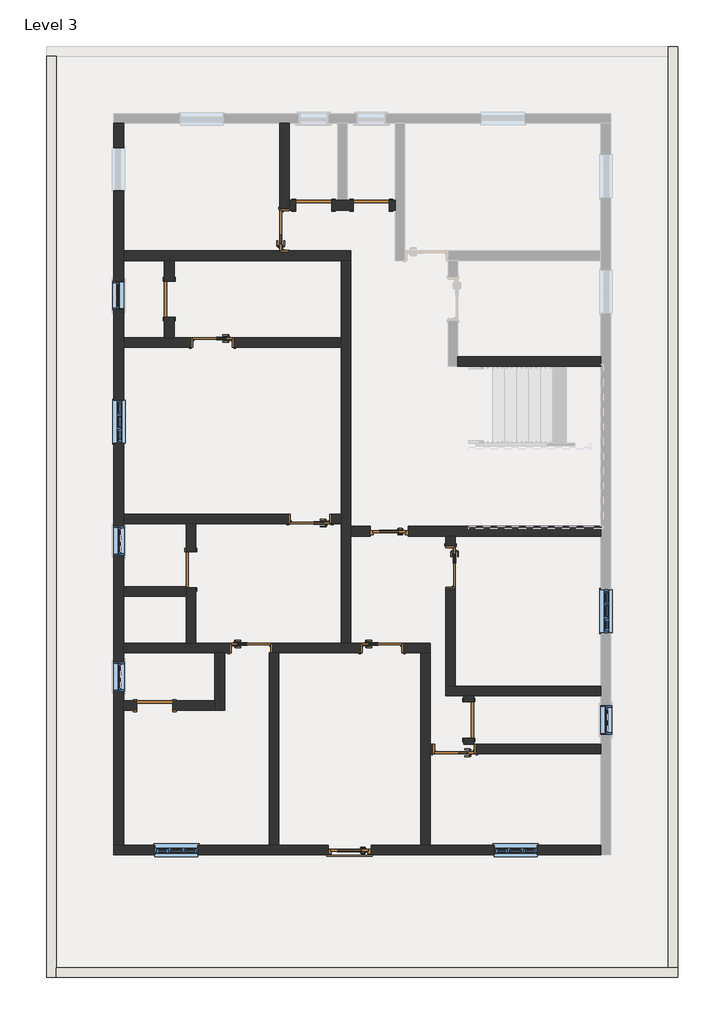
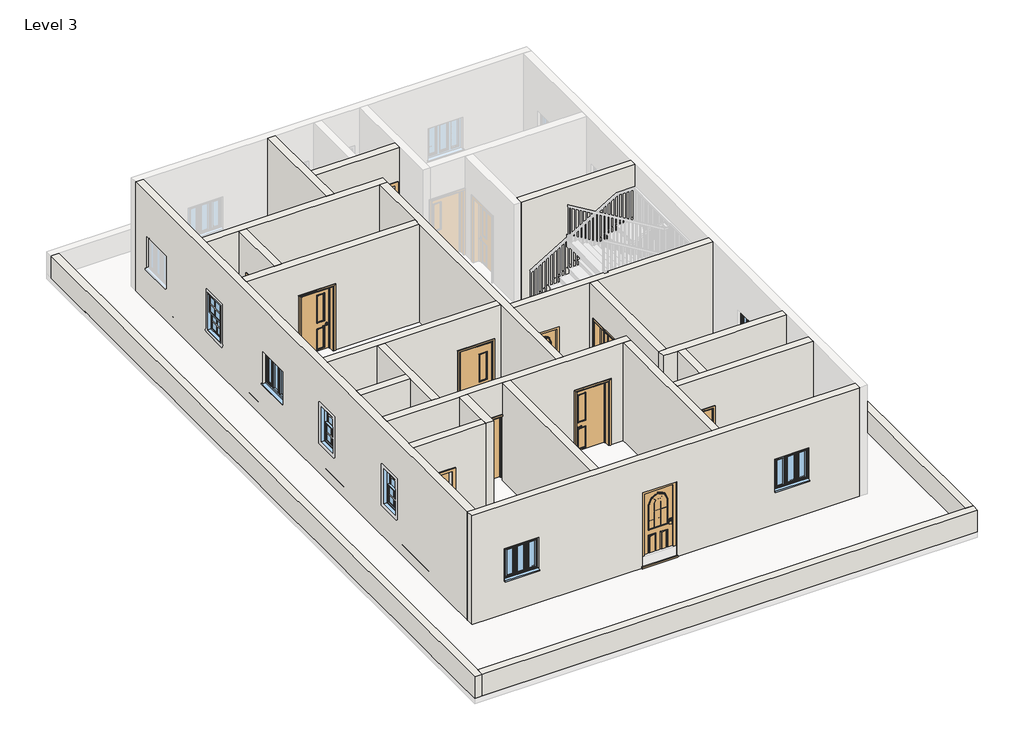
# One storey, part 1 of 3: 25 walls, 15 doors, 8 windows.
"""IFC4 building model written with IfcOpenShell, lengths in millimetres."""

from ifc_helpers import new_model, si_unit, frame, origin, place, context, project, spatial, polyline, outline, extrude, faceted_brep, transform, mapped, element, save
from components import doors_extsgl_w_glazing_bars_arched_810x2110mm_57ea6d9e, doors_extsgl_w_glazing_bars_arched_910x2110mm_1ab485ba, door_aa1d4bf3, door_2f4bc105, door_fadea3f2, door_53b1b562, window_679d2811, windows_tpl_w_glazing_bars_910x910mm_9d987a72

model = new_model("IFC4")

# Units and contexts
model_context = context("Model", 3, world=origin())
ifc_project = project(units=[si_unit("LENGTHUNIT", "METRE", prefix="MILLI")], contexts=[model_context])

# Site, building, storey
site = spatial("IfcSite", under=ifc_project)
building = spatial("IfcBuilding", under=site)
storey = spatial("IfcBuildingStorey", under=building, Name="Level 3", Elevation=6096.0)

# Doors
placement = place(None, origin())
doors_extsgl_w_glazing_bars_arched_810x2110mm_shape = doors_extsgl_w_glazing_bars_arched_810x2110mm_57ea6d9e(model_context)
element("IfcDoor", 1, ObjectType="Doors_ExtSgl_w-Glazing_Bars_Arched : 810x2110mm", at=placement, inside=storey, context=model_context, shape_type="MappedRepresentation", body=[
    mapped(doors_extsgl_w_glazing_bars_arched_810x2110mm_shape, transform((-8090.5711241, 8252.7344295, 6096.0), x_axis=(-1.0, 0.0, 0.0), y_axis=(0.0, -1.0, 0.0), z_axis=(0.0, 0.0, 1.0))),
])
doors_extsgl_w_glazing_bars_arched_910x2110mm_shape = doors_extsgl_w_glazing_bars_arched_910x2110mm_1ab485ba(model_context)
element("IfcDoor", 2, ObjectType="Doors_ExtSgl_w-Glazing_Bars_Arched : 910x2110mm", at=placement, inside=storey, context=model_context, shape_type="MappedRepresentation", body=[
    mapped(doors_extsgl_w_glazing_bars_arched_910x2110mm_shape, transform((-8928.7711241, 1521.7344295, 6096.0), x_axis=(-1.0, 0.0, 0.0), y_axis=(0.0, -1.0, 0.0), z_axis=(0.0, 0.0, 1.0))),
])
door_shape = door_aa1d4bf3(model_context)
element("IfcDoor", 3, ObjectType="Doors_IntSgl_3 : 7'-3\"", at=placement, inside=storey, context=model_context, shape_type="MappedRepresentation", body=[
    mapped(door_shape, transform((-10300.3711241, 14602.7344295, 6096.0), x_axis=(0.0, 1.0, 0.0), y_axis=(-1.0, 0.0, 0.0), z_axis=(0.0, 0.0, 1.0))),
])
element("IfcDoor", 4, ObjectType="Doors_IntSgl_3 : 7'-3\"", at=placement, inside=storey, context=model_context, shape_type="MappedRepresentation", body=[
    mapped(door_shape, transform((-8242.9711241, 5788.9344295, 6096.0), x_axis=(1.0, 0.0, 0.0), y_axis=(0.0, 1.0, 0.0), z_axis=(0.0, 0.0, 1.0))),
])
element("IfcDoor", 5, ObjectType="Doors_IntSgl_3 : 7'-3\"", at=placement, inside=storey, context=model_context, shape_type="MappedRepresentation", body=[
    mapped(door_shape, transform((-6795.1711241, 7490.7344295, 6096.0), x_axis=(0.0, -1.0, 0.0), y_axis=(1.0, 0.0, 0.0), z_axis=(0.0, 0.0, 1.0))),
])
element("IfcDoor", 6, ObjectType="Doors_IntSgl_3 : 7'-3\"", at=placement, inside=storey, context=model_context, shape_type="MappedRepresentation", body=[
    mapped(door_shape, transform((-11011.5711241, 5788.9344295, 6096.0), x_axis=(1.0, 0.0, 0.0), y_axis=(0.0, 1.0, 0.0), z_axis=(0.0, 0.0, 1.0))),
])
element("IfcDoor", 7, ObjectType="Doors_IntSgl_3 : 7'-3\"", at=placement, inside=storey, context=model_context, shape_type="MappedRepresentation", body=[
    mapped(door_shape, transform((-9766.9711241, 8506.7344295, 6096.0), x_axis=(-1.0, 0.0, 0.0), y_axis=(0.0, -1.0, 0.0), z_axis=(0.0, 0.0, 1.0))),
])
element("IfcDoor", 8, ObjectType="Doors_IntSgl_3 : 7'-3\"", at=placement, inside=storey, context=model_context, shape_type="MappedRepresentation", body=[
    mapped(door_shape, transform((-6718.9711241, 3655.3344295, 6096.0), x_axis=(-1.0, 0.0, 0.0), y_axis=(0.0, -1.0, 0.0), z_axis=(0.0, 0.0, 1.0))),
])
door_2_shape = door_2f4bc105(model_context)
element("IfcDoor", 9, ObjectType="Doors_IntSgl_3 : 7'-3\"", at=placement, inside=storey, context=model_context, shape_type="MappedRepresentation", body=[
    mapped(door_2_shape, transform((-11824.3711241, 12240.5344295, 6096.0), x_axis=(-1.0, 0.0, 0.0), y_axis=(0.0, -1.0, 0.0), z_axis=(0.0, 0.0, 1.0))),
])
door_3_shape = door_fadea3f2(model_context)
element("IfcDoor", 10, ObjectType="Single-Flush : 30\" x 80\"", at=placement, inside=storey, context=model_context, shape_type="MappedRepresentation", body=[
    mapped(door_3_shape, transform((-6414.1711241, 4264.9344295, 6096.0), x_axis=(0.0, -1.0, 0.0), y_axis=(1.0, 0.0, 0.0), z_axis=(0.0, 0.0, 1.0))),
])
door_4_shape = door_53b1b562(model_context)
element("IfcDoor", 11, ObjectType="Single-Flush : 30\" x 80\"", at=placement, inside=storey, context=model_context, shape_type="MappedRepresentation", body=[
    mapped(door_4_shape, transform((-13043.5711241, 4569.7344295, 6096.0), x_axis=(-1.0, 0.0, 0.0), y_axis=(0.0, -1.0, 0.0), z_axis=(0.0, 0.0, 1.0))),
])
element("IfcDoor", 12, ObjectType="Single-Flush : 30\" x 80\"", at=placement, inside=storey, context=model_context, shape_type="MappedRepresentation", body=[
    mapped(door_4_shape, transform((-12281.5711241, 7439.9344295, 6096.0), x_axis=(0.0, -1.0, 0.0), y_axis=(1.0, 0.0, 0.0), z_axis=(0.0, 0.0, 1.0))),
])
element("IfcDoor", 13, ObjectType="Single-Flush : 30\" x 80\"", at=placement, inside=storey, context=model_context, shape_type="MappedRepresentation", body=[
    mapped(door_4_shape, transform((-12738.7711241, 13154.9344295, 6096.0), x_axis=(0.0, -1.0, 0.0), y_axis=(1.0, 0.0, 0.0), z_axis=(0.0, 0.0, 1.0))),
])
element("IfcDoor", 14, ObjectType="Single-Flush : 30\" x 80\"", at=placement, inside=storey, context=model_context, shape_type="MappedRepresentation", body=[
    mapped(door_4_shape, transform((-9690.7711241, 15136.1344295, 6096.0), x_axis=(-1.0, 0.0, 0.0), y_axis=(0.0, -1.0, 0.0), z_axis=(0.0, 0.0, 1.0))),
])
element("IfcDoor", 15, ObjectType="Single-Flush : 30\" x 80\"", at=placement, inside=storey, context=model_context, shape_type="MappedRepresentation", body=[
    mapped(door_4_shape, transform((-8471.5711241, 15136.1344295, 6096.0), x_axis=(-1.0, 0.0, 0.0), y_axis=(0.0, -1.0, 0.0), z_axis=(0.0, 0.0, 1.0))),
])

# Walls
element("IfcWall", 16, ObjectType="Generic -4.5\" p", at=placement, inside=storey, context=model_context, shape_type="Brep", body=[
    faceted_brep([(-10401.9711241, 14170.9344295, 9144.0), (-10401.9711241, 16863.3344295, 9144.0), (-10401.9711241, 16863.3344295, 6096.0), (-10401.9711241, 15059.9344295, 6096.0), (-10401.9711241, 15059.9344295, 8229.6), (-10401.9711241, 14170.9344295, 8229.6), (-10198.7711241, 16863.3344295, 9144.0), (-10198.7711241, 15237.7344295, 9144.0), (-10198.7711241, 15034.5344295, 9144.0), (-10198.7711241, 14170.9344295, 9144.0), (-10198.7711241, 14170.9344295, 8229.6), (-10198.7711241, 15059.9344295, 8229.6), (-10198.7711241, 15059.9344295, 6096.0), (-10198.7711241, 15237.7344295, 6096.0), (-10198.7711241, 16863.3344295, 6096.0)], [[[0, 1, 2, 3, 4, 5]], [[6, 7, 8, 9, 10, 11, 12, 13, 14]], [[2, 14, 13, 12, 3]], [[1, 0, 9, 8, 7, 6]], [[2, 1, 6, 14]], [[9, 0, 5, 10]], [[11, 4, 3, 12]], [[4, 11, 10, 5]]]),
])
element("IfcWall", 17, ObjectType="Generic -4.5\" p", at=placement, inside=storey, context=model_context, shape_type="Brep", body=[
    faceted_brep([(-9309.7711241, 15034.5344295, 6096.0), (-8852.5711241, 15034.5344295, 6096.0), (-8852.5711241, 15034.5344295, 8128.0), (-8090.5711241, 15034.5344295, 8128.0), (-8090.5711241, 15034.5344295, 6096.0), (-7963.5711241, 15034.5344295, 6096.0), (-7963.5711241, 15034.5344295, 9144.0), (-10198.7711241, 15034.5344295, 9144.0), (-10198.7711241, 15034.5344295, 6096.0), (-10071.7711241, 15034.5344295, 6096.0), (-10071.7711241, 15034.5344295, 8128.0), (-9309.7711241, 15034.5344295, 8128.0), (-8852.5711241, 15237.7344295, 8128.0), (-8852.5711241, 15237.7344295, 6096.0), (-8979.5711241, 15237.7344295, 6096.0), (-9182.7711241, 15237.7344295, 6096.0), (-9309.7711241, 15237.7344295, 6096.0), (-9309.7711241, 15237.7344295, 8128.0), (-10071.7711241, 15237.7344295, 8128.0), (-10071.7711241, 15237.7344295, 6096.0), (-10198.7711241, 15237.7344295, 6096.0), (-10198.7711241, 15237.7344295, 9144.0), (-9182.7711241, 15237.7344295, 9144.0), (-8979.5711241, 15237.7344295, 9144.0), (-7963.5711241, 15237.7344295, 9144.0), (-7963.5711241, 15237.7344295, 6096.0), (-8090.5711241, 15237.7344295, 6096.0), (-8090.5711241, 15237.7344295, 8128.0), (-10198.7711241, 15059.9344295, 6096.0)], [[[0, 1, 2, 3, 4, 5, 6, 7, 8, 9, 10, 11]], [[12, 13, 14, 15, 16, 17, 18, 19, 20, 21, 22, 23, 24, 25, 26, 27]], [[20, 19, 9, 8, 28]], [[26, 25, 5, 4]], [[16, 15, 14, 13, 1, 0]], [[7, 6, 24, 23, 22, 21]], [[8, 7, 21, 20, 28]], [[6, 5, 25, 24]], [[10, 9, 19, 18]], [[11, 10, 18, 17]], [[0, 11, 17, 16]], [[2, 1, 13, 12]], [[3, 2, 12, 27]], [[4, 3, 27, 26]]]),
])
element("IfcWall", 18, ObjectType="Generic -4.5\" p", at=placement, inside=storey, context=model_context, shape_type="Brep", body=[
    faceted_brep([(-13703.9711241, 13967.7344295, 6096.0), (-12840.3711241, 13967.7344295, 6096.0), (-12637.1711241, 13967.7344295, 6096.0), (-9106.5711241, 13967.7344295, 6096.0), (-8903.3711241, 13967.7344295, 6096.0), (-8903.3711241, 13967.7344295, 9144.0), (-9106.5711241, 13967.7344295, 9144.0), (-12637.1711241, 13967.7344295, 9144.0), (-12840.3711241, 13967.7344295, 9144.0), (-13703.9711241, 13967.7344295, 9144.0), (-13703.9711241, 14170.9344295, 9144.0), (-10401.9711241, 14170.9344295, 9144.0), (-10198.7711241, 14170.9344295, 9144.0), (-8903.3711241, 14170.9344295, 9144.0), (-8903.3711241, 14170.9344295, 6096.0), (-10198.7711241, 14170.9344295, 6096.0), (-10198.7711241, 14170.9344295, 8229.6), (-10401.9711241, 14170.9344295, 8229.6), (-10401.9711241, 14170.9344295, 6096.0), (-13703.9711241, 14170.9344295, 6096.0), (-10401.9711241, 14145.5344295, 6096.0), (-10198.7711241, 14145.5344295, 6096.0), (-10198.7711241, 14145.5344295, 8229.6), (-10401.9711241, 14145.5344295, 8229.6)], [[[0, 1, 2, 3, 4, 5, 6, 7, 8, 9]], [[10, 11, 12, 13, 14, 15, 16, 17, 18, 19]], [[4, 3, 2, 1, 0, 19, 18, 20, 21, 15, 14]], [[9, 8, 7, 6, 5, 13, 12, 11, 10]], [[0, 9, 10, 19]], [[5, 4, 14, 13]], [[21, 22, 16, 15]], [[23, 20, 18, 17]], [[22, 23, 17, 16]], [[22, 21, 20, 23]]]),
])
element("IfcWall", 19, ObjectType="Generic -4.5\" p", at=placement, inside=storey, context=model_context, shape_type="Brep", body=[
    faceted_brep([(-9106.5711241, 13967.7344295, 6096.0), (-9106.5711241, 12342.1344295, 6096.0), (-9106.5711241, 12138.9344295, 6096.0), (-9106.5711241, 8608.3344295, 6096.0), (-9106.5711241, 8405.1344295, 6096.0), (-9106.5711241, 5890.5344295, 6096.0), (-9106.5711241, 5890.5344295, 9144.0), (-9106.5711241, 8405.1344295, 9144.0), (-9106.5711241, 8608.3344295, 9144.0), (-9106.5711241, 12138.9344295, 9144.0), (-9106.5711241, 12342.1344295, 9144.0), (-9106.5711241, 13967.7344295, 9144.0), (-8903.3711241, 13967.7344295, 6096.0), (-8903.3711241, 13967.7344295, 9144.0), (-8903.3711241, 8354.3344295, 9144.0), (-8903.3711241, 8151.1344295, 9144.0), (-8903.3711241, 5890.5344295, 9144.0), (-8903.3711241, 5890.5344295, 6096.0), (-8903.3711241, 8151.1344295, 6096.0), (-8903.3711241, 8354.3344295, 6096.0)], [[[0, 1, 2, 3, 4, 5, 6, 7, 8, 9, 10, 11]], [[12, 13, 14, 15, 16, 17, 18, 19]], [[5, 4, 3, 2, 1, 0, 12, 19, 18, 17]], [[11, 10, 9, 8, 7, 6, 16, 15, 14, 13]], [[0, 11, 13, 12]], [[6, 5, 17, 16]]]),
])
element("IfcWall", 20, ObjectType="Generic -4.5\" p", at=placement, inside=storey, context=model_context, shape_type="Brep", body=[
    faceted_brep([(-13703.9711241, 12342.1344295, 9144.0), (-12840.3711241, 12342.1344295, 9144.0), (-12637.1711241, 12342.1344295, 9144.0), (-9106.5711241, 12342.1344295, 9144.0), (-9106.5711241, 12342.1344295, 6096.0), (-11367.1711241, 12342.1344295, 6096.0), (-11367.1711241, 12342.1344295, 8229.6), (-12281.5711241, 12342.1344295, 8229.6), (-12281.5711241, 12342.1344295, 6096.0), (-12637.1711241, 12342.1344295, 6096.0), (-12840.3711241, 12342.1344295, 6096.0), (-13703.9711241, 12342.1344295, 6096.0), (-9106.5711241, 12138.9344295, 9144.0), (-13703.9711241, 12138.9344295, 9144.0), (-13703.9711241, 12138.9344295, 6096.0), (-12281.5711241, 12138.9344295, 6096.0), (-12281.5711241, 12138.9344295, 8229.6), (-11367.1711241, 12138.9344295, 8229.6), (-11367.1711241, 12138.9344295, 6096.0), (-9106.5711241, 12138.9344295, 6096.0)], [[[0, 1, 2, 3, 4, 5, 6, 7, 8, 9, 10, 11]], [[12, 13, 14, 15, 16, 17, 18, 19]], [[4, 19, 18, 5]], [[14, 11, 10, 9, 8, 15]], [[3, 2, 1, 0, 13, 12]], [[4, 3, 12, 19]], [[0, 11, 14, 13]], [[7, 16, 15, 8]], [[16, 7, 6, 17]], [[17, 6, 5, 18]]]),
])
element("IfcWall", 21, ObjectType="Generic -4.5\" p", at=placement, inside=storey, context=model_context, shape_type="SweptSolid", body=[
    extrude(outline(polyline([(12773.9344295, 8128.0), (12773.9344295, 6096.0), (12342.1344295, 6096.0), (12342.1344295, 9144.0), (13967.7344295, 9144.0), (13967.7344295, 6096.0), (13535.9344295, 6096.0), (13535.9344295, 8128.0), (12773.9344295, 8128.0)])), frame((-12840.3711241, 0.0, 0.0), z_axis=(1.0, 0.0, 0.0), x_axis=(0.0, 1.0, 0.0)), (0.0, 0.0, 1.0), 203.2),
])
element("IfcWall", 22, ObjectType="Generic -4.5\" p", at=placement, inside=storey, context=model_context, shape_type="Brep", body=[
    faceted_brep([(-9106.5711241, 8405.1344295, 9144.0), (-12179.9711241, 8405.1344295, 9144.0), (-12383.1711241, 8405.1344295, 9144.0), (-13703.9711241, 8405.1344295, 9144.0), (-13703.9711241, 8405.1344295, 6096.0), (-12383.1711241, 8405.1344295, 6096.0), (-12179.9711241, 8405.1344295, 6096.0), (-10224.1711241, 8405.1344295, 6096.0), (-10224.1711241, 8405.1344295, 8229.6), (-9309.7711241, 8405.1344295, 8229.6), (-9309.7711241, 8405.1344295, 6096.0), (-9106.5711241, 8405.1344295, 6096.0), (-13703.9711241, 8608.3344295, 9144.0), (-9106.5711241, 8608.3344295, 9144.0), (-9106.5711241, 8608.3344295, 6096.0), (-9309.7711241, 8608.3344295, 6096.0), (-9309.7711241, 8608.3344295, 8229.6), (-10224.1711241, 8608.3344295, 8229.6), (-10224.1711241, 8608.3344295, 6096.0), (-13703.9711241, 8608.3344295, 6096.0)], [[[0, 1, 2, 3, 4, 5, 6, 7, 8, 9, 10, 11]], [[12, 13, 14, 15, 16, 17, 18, 19]], [[4, 19, 18, 7, 6, 5]], [[14, 11, 10, 15]], [[3, 2, 1, 0, 13, 12]], [[4, 3, 12, 19]], [[0, 11, 14, 13]], [[17, 8, 7, 18]], [[8, 17, 16, 9]], [[9, 16, 15, 10]]]),
])
element("IfcWall", 23, ObjectType="Generic -4.5\" p", at=placement, inside=storey, context=model_context, shape_type="Brep", body=[
    faceted_brep([(-12383.1711241, 7058.9344295, 8128.0), (-12383.1711241, 7058.9344295, 6096.0), (-12383.1711241, 6881.1344295, 6096.0), (-12383.1711241, 5890.5344295, 6096.0), (-12383.1711241, 5890.5344295, 9144.0), (-12383.1711241, 6881.1344295, 9144.0), (-12383.1711241, 7084.3344295, 9144.0), (-12383.1711241, 8405.1344295, 9144.0), (-12383.1711241, 8405.1344295, 6096.0), (-12383.1711241, 7820.9344295, 6096.0), (-12383.1711241, 7820.9344295, 8128.0), (-12179.9711241, 5890.5344295, 6096.0), (-12179.9711241, 7058.9344295, 6096.0), (-12179.9711241, 7058.9344295, 8128.0), (-12179.9711241, 7820.9344295, 8128.0), (-12179.9711241, 7820.9344295, 6096.0), (-12179.9711241, 8405.1344295, 6096.0), (-12179.9711241, 8405.1344295, 9144.0), (-12179.9711241, 5890.5344295, 9144.0)], [[[0, 1, 2, 3, 4, 5, 6, 7, 8, 9, 10]], [[11, 12, 13, 14, 15, 16, 17, 18]], [[9, 8, 16, 15]], [[3, 2, 1, 12, 11]], [[7, 6, 5, 4, 18, 17]], [[8, 7, 17, 16]], [[4, 3, 11, 18]], [[13, 12, 1, 0]], [[14, 13, 0, 10]], [[15, 14, 10, 9]]]),
])
element("IfcWall", 24, ObjectType="Generic -4.5\" p", at=placement, inside=storey, context=model_context, shape_type="Brep", body=[
    faceted_brep([(-13703.9711241, 6881.1344295, 6096.0), (-12383.1711241, 6881.1344295, 6096.0), (-12383.1711241, 6881.1344295, 9144.0), (-13703.9711241, 6881.1344295, 9144.0), (-13703.9711241, 7084.3344295, 6096.0), (-13703.9711241, 7084.3344295, 9144.0), (-12383.1711241, 7084.3344295, 9144.0), (-12383.1711241, 7084.3344295, 6096.0), (-12383.1711241, 7058.9344295, 6096.0)], [[[0, 1, 2, 3]], [[4, 5, 6, 7]], [[1, 0, 4, 7, 8]], [[3, 2, 6, 5]], [[0, 3, 5, 4]], [[2, 1, 8, 7, 6]]]),
])
element("IfcWall", 25, ObjectType="Generic -4.5\" p", at=placement, inside=storey, context=model_context, shape_type="Brep", body=[
    faceted_brep([(-7226.9711241, 5687.3344295, 9144.0), (-7430.1711241, 5687.3344295, 9144.0), (-10427.3711241, 5687.3344295, 9144.0), (-10630.5711241, 5687.3344295, 9144.0), (-11570.3711241, 5687.3344295, 9144.0), (-11773.5711241, 5687.3344295, 9144.0), (-13703.9711241, 5687.3344295, 9144.0), (-13703.9711241, 5687.3344295, 6096.0), (-11773.5711241, 5687.3344295, 6096.0), (-11570.3711241, 5687.3344295, 6096.0), (-11468.7711241, 5687.3344295, 6096.0), (-11468.7711241, 5687.3344295, 8229.6), (-10554.3711241, 5687.3344295, 8229.6), (-10554.3711241, 5687.3344295, 6096.0), (-10427.3711241, 5687.3344295, 6096.0), (-8700.1711241, 5687.3344295, 6096.0), (-8700.1711241, 5687.3344295, 8229.6), (-7785.7711241, 5687.3344295, 8229.6), (-7785.7711241, 5687.3344295, 6096.0), (-7430.1711241, 5687.3344295, 6096.0), (-7226.9711241, 5687.3344295, 6096.0), (-13703.9711241, 5890.5344295, 9144.0), (-12383.1711241, 5890.5344295, 9144.0), (-12179.9711241, 5890.5344295, 9144.0), (-9106.5711241, 5890.5344295, 9144.0), (-8903.3711241, 5890.5344295, 9144.0), (-7226.9711241, 5890.5344295, 9144.0), (-7226.9711241, 5890.5344295, 6096.0), (-7785.7711241, 5890.5344295, 6096.0), (-7785.7711241, 5890.5344295, 8229.6), (-8700.1711241, 5890.5344295, 8229.6), (-8700.1711241, 5890.5344295, 6096.0), (-8903.3711241, 5890.5344295, 6096.0), (-9106.5711241, 5890.5344295, 6096.0), (-10554.3711241, 5890.5344295, 6096.0), (-10554.3711241, 5890.5344295, 8229.6), (-11468.7711241, 5890.5344295, 8229.6), (-11468.7711241, 5890.5344295, 6096.0), (-12179.9711241, 5890.5344295, 6096.0), (-12383.1711241, 5890.5344295, 6096.0), (-13703.9711241, 5890.5344295, 6096.0)], [[[0, 1, 2, 3, 4, 5, 6, 7, 8, 9, 10, 11, 12, 13, 14, 15, 16, 17, 18, 19, 20]], [[21, 22, 23, 24, 25, 26, 27, 28, 29, 30, 31, 32, 33, 34, 35, 36, 37, 38, 39, 40]], [[7, 40, 39, 38, 37, 10, 9, 8]], [[27, 20, 19, 18, 28]], [[31, 15, 14, 13, 34, 33, 32]], [[6, 5, 4, 3, 2, 1, 0, 26, 25, 24, 23, 22, 21]], [[7, 6, 21, 40]], [[0, 20, 27, 26]], [[17, 29, 28, 18]], [[29, 17, 16, 30]], [[30, 16, 15, 31]], [[12, 35, 34, 13]], [[35, 12, 11, 36]], [[36, 11, 10, 37]]]),
])
element("IfcWall", 26, ObjectType="Generic -4.5\" p", at=placement, inside=storey, context=model_context, shape_type="Brep", body=[
    faceted_brep([(-7430.1711241, 5687.3344295, 6096.0), (-7430.1711241, 1623.3344295, 6096.0), (-7430.1711241, 1623.3344295, 9144.0), (-7430.1711241, 5687.3344295, 9144.0), (-7226.9711241, 5687.3344295, 6096.0), (-7226.9711241, 5687.3344295, 9144.0), (-7226.9711241, 3756.9344295, 9144.0), (-7226.9711241, 3553.7344295, 9144.0), (-7226.9711241, 1623.3344295, 9144.0), (-7226.9711241, 1623.3344295, 6096.0), (-7226.9711241, 3553.7344295, 6096.0), (-7226.9711241, 3756.9344295, 6096.0)], [[[0, 1, 2, 3]], [[4, 5, 6, 7, 8, 9, 10, 11]], [[1, 0, 4, 11, 10, 9]], [[3, 2, 8, 7, 6, 5]], [[0, 3, 5, 4]], [[2, 1, 9, 8]]]),
])
element("IfcWall", 27, ObjectType="Generic -4.5\" p", at=placement, inside=storey, context=model_context, shape_type="Brep", body=[
    faceted_brep([(-11773.5711241, 5687.3344295, 6096.0), (-11773.5711241, 4671.3344295, 6096.0), (-11773.5711241, 4468.1344295, 6096.0), (-11773.5711241, 4468.1344295, 9144.0), (-11773.5711241, 4671.3344295, 9144.0), (-11773.5711241, 5687.3344295, 9144.0), (-11570.3711241, 5687.3344295, 6096.0), (-11570.3711241, 5687.3344295, 9144.0), (-11570.3711241, 4468.1344295, 9144.0), (-11570.3711241, 4468.1344295, 6096.0)], [[[0, 1, 2, 3, 4, 5]], [[6, 7, 8, 9]], [[2, 1, 0, 6, 9]], [[5, 4, 3, 8, 7]], [[0, 5, 7, 6]], [[3, 2, 9, 8]]]),
])
element("IfcWall", 28, ObjectType="Generic -4.5\" p", at=placement, inside=storey, context=model_context, shape_type="SweptSolid", body=[
    extrude(outline(polyline([(6096.0, -13703.9711241), (6096.0, -13424.5711241), (8128.0, -13424.5711241), (8128.0, -12662.5711241), (6096.0, -12662.5711241), (6096.0, -11773.5711241), (9144.0, -11773.5711241), (9144.0, -13703.9711241), (6096.0, -13703.9711241)])), frame((0.0, 4468.1344295, 0.0), z_axis=(0.0, 1.0, 0.0), x_axis=(0.0, 0.0, 1.0)), (0.0, 0.0, 1.0), 203.2),
])
element("IfcWall", 29, ObjectType="Generic -4.5\" p", at=placement, inside=storey, context=model_context, shape_type="Brep", body=[
    faceted_brep([(-10630.5711241, 5687.3344295, 6096.0), (-10630.5711241, 1623.3344295, 6096.0), (-10630.5711241, 1623.3344295, 9144.0), (-10630.5711241, 5687.3344295, 9144.0), (-10427.3711241, 5687.3344295, 6096.0), (-10427.3711241, 5687.3344295, 9144.0), (-10427.3711241, 1623.3344295, 9144.0), (-10427.3711241, 1623.3344295, 6096.0), (-10554.3711241, 5687.3344295, 6096.0)], [[[0, 1, 2, 3]], [[4, 5, 6, 7]], [[1, 0, 8, 4, 7]], [[3, 2, 6, 5]], [[2, 1, 7, 6]], [[0, 3, 5, 4, 8]]]),
])
element("IfcWall", 30, ObjectType="Generic -4.5\" p", at=placement, inside=storey, context=model_context, shape_type="Brep", body=[
    faceted_brep([(-3620.1711241, 3553.7344295, 9144.0), (-7226.9711241, 3553.7344295, 9144.0), (-7226.9711241, 3553.7344295, 6096.0), (-7176.1711241, 3553.7344295, 6096.0), (-7176.1711241, 3553.7344295, 8229.6), (-6261.7711241, 3553.7344295, 8229.6), (-6261.7711241, 3553.7344295, 6096.0), (-3620.1711241, 3553.7344295, 6096.0), (-7226.9711241, 3756.9344295, 9144.0), (-6515.7711241, 3756.9344295, 9144.0), (-6312.5711241, 3756.9344295, 9144.0), (-3620.1711241, 3756.9344295, 9144.0), (-3620.1711241, 3756.9344295, 6096.0), (-6261.7711241, 3756.9344295, 6096.0), (-6261.7711241, 3756.9344295, 8229.6), (-7176.1711241, 3756.9344295, 8229.6), (-7176.1711241, 3756.9344295, 6096.0), (-7226.9711241, 3756.9344295, 6096.0)], [[[0, 1, 2, 3, 4, 5, 6, 7]], [[8, 9, 10, 11, 12, 13, 14, 15, 16, 17]], [[2, 17, 16, 3]], [[12, 7, 6, 13]], [[1, 0, 11, 10, 9, 8]], [[0, 7, 12, 11]], [[2, 1, 8, 17]], [[15, 4, 3, 16]], [[4, 15, 14, 5]], [[5, 14, 13, 6]]]),
])
element("IfcWall", 31, ObjectType="Generic -4.5\" p", at=placement, inside=storey, context=model_context, shape_type="SweptSolid", body=[
    extrude(outline(polyline([(3883.9344295, 8128.0), (3883.9344295, 6096.0), (3756.9344295, 6096.0), (3756.9344295, 9144.0), (4772.9344295, 9144.0), (4772.9344295, 6096.0), (4645.9344295, 6096.0), (4645.9344295, 8128.0), (3883.9344295, 8128.0)])), frame((-6515.7711241, 0.0, 0.0), z_axis=(1.0, 0.0, 0.0), x_axis=(0.0, 1.0, 0.0)), (0.0, 0.0, 1.0), 203.2),
])
element("IfcWall", 32, ObjectType="Generic -4.5\" p", at=placement, inside=storey, context=model_context, shape_type="Brep", body=[
    faceted_brep([(-3620.1711241, 4976.1344295, 6096.0), (-6693.5711241, 4976.1344295, 6096.0), (-6896.7711241, 4976.1344295, 6096.0), (-6896.7711241, 4976.1344295, 9144.0), (-6693.5711241, 4976.1344295, 9144.0), (-3620.1711241, 4976.1344295, 9144.0), (-3620.1711241, 4772.9344295, 6096.0), (-3620.1711241, 4772.9344295, 9144.0), (-6312.5711241, 4772.9344295, 9144.0), (-6515.7711241, 4772.9344295, 9144.0), (-6896.7711241, 4772.9344295, 9144.0), (-6896.7711241, 4772.9344295, 6096.0), (-6515.7711241, 4772.9344295, 6096.0), (-6312.5711241, 4772.9344295, 6096.0)], [[[0, 1, 2, 3, 4, 5]], [[6, 7, 8, 9, 10, 11, 12, 13]], [[2, 1, 0, 6, 13, 12, 11]], [[5, 4, 3, 10, 9, 8, 7]], [[0, 5, 7, 6]], [[3, 2, 11, 10]]]),
])
element("IfcWall", 33, ObjectType="Generic -4.5\" p", at=placement, inside=storey, context=model_context, shape_type="SweptSolid", body=[
    extrude(outline(polyline([(4976.1344295, 9144.0), (8151.1344295, 9144.0), (8151.1344295, 6096.0), (7947.9344295, 6096.0), (7947.9344295, 8229.6), (7033.5344295, 8229.6), (7033.5344295, 6096.0), (4976.1344295, 6096.0), (4976.1344295, 9144.0)])), frame((-6896.7711241, 0.0, 0.0), z_axis=(1.0, 0.0, 0.0), x_axis=(0.0, 1.0, 0.0)), (0.0, 0.0, 1.0), 203.2),
])
element("IfcWall", 34, ObjectType="Generic -4.5\" p", at=placement, inside=storey, context=model_context, shape_type="SweptSolid", body=[
    extrude(outline(polyline([(-3620.1711241, 11732.5344295), (-6642.7711241, 11732.5344295), (-6642.7711241, 11935.7344295), (-3620.1711241, 11935.7344295), (-3620.1711241, 11732.5344295)])), frame((0.0, 0.0, 6096.0), z_axis=(0.0, 0.0, 1.0), x_axis=(1.0, 0.0, 0.0)), (0.0, 0.0, 1.0), 3048.0),
])
element("IfcWall", 35, ObjectType="Generic -4.5\" p", at=placement, inside=storey, context=model_context, shape_type="Brep", body=[
    faceted_brep([(-8495.5711241, 8354.3344295, 8206.0), (-8495.5711241, 8354.3344295, 6096.0), (-8903.3711241, 8354.3344295, 6096.0), (-8903.3711241, 8354.3344295, 9144.0), (-3620.1711241, 8354.3344295, 9144.0), (-3620.1711241, 8354.3344295, 6096.0), (-7685.5711241, 8354.3344295, 6096.0), (-7685.5711241, 8354.3344295, 8206.0), (-8903.3711241, 8151.1344295, 6096.0), (-8495.5711241, 8151.1344295, 6096.0), (-8495.5711241, 8151.1344295, 8206.0), (-7685.5711241, 8151.1344295, 8206.0), (-7685.5711241, 8151.1344295, 6096.0), (-6896.7711241, 8151.1344295, 6096.0), (-6693.5711241, 8151.1344295, 6096.0), (-3620.1711241, 8151.1344295, 6096.0), (-3620.1711241, 8151.1344295, 9144.0), (-6693.5711241, 8151.1344295, 9144.0), (-6896.7711241, 8151.1344295, 9144.0), (-8903.3711241, 8151.1344295, 9144.0)], [[[0, 1, 2, 3, 4, 5, 6, 7]], [[8, 9, 10, 11, 12, 13, 14, 15, 16, 17, 18, 19]], [[6, 5, 15, 14, 13, 12]], [[2, 1, 9, 8]], [[4, 3, 19, 18, 17, 16]], [[5, 4, 16, 15]], [[3, 2, 8, 19]], [[12, 11, 7, 6]], [[10, 9, 1, 0]], [[11, 10, 0, 7]]]),
])
element("IfcWall", 36, ObjectType="Generic -4.5\" p", at=placement, inside=storey, context=model_context, shape_type="Brep", body=[
    faceted_brep([(-15126.3711241, -1171.3990222, 6096.0), (-15126.3711241, -968.1990222, 6096.0), (-15126.3711241, 18285.0009778, 6096.0), (-15126.3711241, 18285.0009778, 6705.6), (-15126.3711241, -968.1990222, 6705.6), (-15126.3711241, -1171.3990222, 6705.6), (-15329.5711241, -1171.3990222, 6096.0), (-15329.5711241, -1171.3990222, 6705.6), (-15329.5711241, 18285.0009778, 6705.6), (-15329.5711241, 18285.0009778, 6096.0)], [[[0, 1, 2, 3, 4, 5]], [[6, 7, 8, 9]], [[2, 1, 0, 6, 9]], [[5, 4, 3, 8, 7]], [[0, 5, 7, 6]], [[3, 2, 9, 8]]]),
])
element("IfcWall", 37, ObjectType="Generic -4.5\" p", at=placement, inside=storey, context=model_context, shape_type="Brep", body=[
    faceted_brep([(-1994.5711241, -968.1990222, 6096.0), (-2197.7711241, -968.1990222, 6096.0), (-15126.3711241, -968.1990222, 6096.0), (-15126.3711241, -968.1990222, 6705.6), (-2197.7711241, -968.1990222, 6705.6), (-1994.5711241, -968.1990222, 6705.6), (-1994.5711241, -1171.3990222, 6096.0), (-1994.5711241, -1171.3990222, 6705.6), (-15126.3711241, -1171.3990222, 6705.6), (-15126.3711241, -1171.3990222, 6096.0)], [[[0, 1, 2, 3, 4, 5]], [[6, 7, 8, 9]], [[2, 1, 0, 6, 9]], [[5, 4, 3, 8, 7]], [[0, 5, 7, 6]], [[3, 2, 9, 8]]]),
])
element("IfcWall", 38, ObjectType="Generic -4.5\" p", at=placement, inside=storey, context=model_context, shape_type="Brep", body=[
    faceted_brep([(-2197.7711241, 18488.2009778, 6096.0), (-2197.7711241, 18285.0009778, 6096.0), (-2197.7711241, -968.1990222, 6096.0), (-2197.7711241, -968.1990222, 6705.6), (-2197.7711241, 18285.0009778, 6705.6), (-2197.7711241, 18488.2009778, 6705.6), (-1994.5711241, 18488.2009778, 6096.0), (-1994.5711241, 18488.2009778, 6705.6), (-1994.5711241, -968.1990222, 6705.6), (-1994.5711241, -968.1990222, 6096.0)], [[[0, 1, 2, 3, 4, 5]], [[6, 7, 8, 9]], [[2, 1, 0, 6, 9]], [[5, 4, 3, 8, 7]], [[0, 5, 7, 6]], [[3, 2, 9, 8]]]),
])
element("IfcWall", 39, ObjectType="Generic -9\" w", at=placement, inside=storey, context=model_context, shape_type="Brep", body=[
    faceted_brep([(-9383.7711241, 1623.3344295, 8206.0), (-9383.7711241, 1623.3344295, 6096.0), (-10427.3711241, 1623.3344295, 6096.0), (-10630.5711241, 1623.3344295, 6096.0), (-13703.9711241, 1623.3344295, 6096.0), (-13907.1711241, 1623.3344295, 6096.0), (-13907.1711241, 1623.3344295, 9144.0), (-13703.9711241, 1623.3344295, 9144.0), (-10630.5711241, 1623.3344295, 9144.0), (-10427.3711241, 1623.3344295, 9144.0), (-7430.1711241, 1623.3344295, 9144.0), (-7226.9711241, 1623.3344295, 9144.0), (-3620.1711241, 1623.3344295, 9144.0), (-3620.1711241, 1623.3344295, 6096.0), (-7226.9711241, 1623.3344295, 6096.0), (-7430.1711241, 1623.3344295, 6096.0), (-8473.7711241, 1623.3344295, 6096.0), (-8473.7711241, 1623.3344295, 8206.0), (-12131.3711241, 1623.3344295, 7920.4), (-13041.3711241, 1623.3344295, 7920.4), (-13041.3711241, 1623.3344295, 7010.4), (-12131.3711241, 1623.3344295, 7010.4), (-4968.5711241, 1623.3344295, 7920.4), (-5878.5711241, 1623.3344295, 7920.4), (-5878.5711241, 1623.3344295, 7010.4), (-4968.5711241, 1623.3344295, 7010.4), (-13907.1711241, 1420.1344295, 6096.0), (-9383.7711241, 1420.1344295, 6096.0), (-9383.7711241, 1420.1344295, 8206.0), (-8473.7711241, 1420.1344295, 8206.0), (-8473.7711241, 1420.1344295, 6096.0), (-3620.1711241, 1420.1344295, 6096.0), (-3620.1711241, 1420.1344295, 9144.0), (-13907.1711241, 1420.1344295, 9144.0), (-12131.3711241, 1420.1344295, 7920.4), (-12131.3711241, 1420.1344295, 7010.4), (-13041.3711241, 1420.1344295, 7010.4), (-13041.3711241, 1420.1344295, 7920.4), (-4968.5711241, 1420.1344295, 7920.4), (-4968.5711241, 1420.1344295, 7010.4), (-5878.5711241, 1420.1344295, 7010.4), (-5878.5711241, 1420.1344295, 7920.4)], [[[0, 1, 2, 3, 4, 5, 6, 7, 8, 9, 10, 11, 12, 13, 14, 15, 16, 17], [18, 19, 20, 21], [22, 23, 24, 25]], [[26, 27, 28, 29, 30, 31, 32, 33], [34, 35, 36, 37], [38, 39, 40, 41]], [[5, 4, 3, 2, 1, 27, 26]], [[16, 15, 14, 13, 31, 30]], [[12, 11, 10, 9, 8, 7, 6, 33, 32]], [[13, 12, 32, 31]], [[6, 5, 26, 33]], [[30, 29, 17, 16]], [[28, 27, 1, 0]], [[29, 28, 0, 17]], [[35, 34, 18, 21]], [[36, 35, 21, 20]], [[37, 36, 20, 19]], [[34, 37, 19, 18]], [[39, 38, 22, 25]], [[40, 39, 25, 24]], [[41, 40, 24, 23]], [[38, 41, 23, 22]]]),
])
element("IfcWall", 40, ObjectType="Generic -9\" w", at=placement, inside=storey, context=model_context, shape_type="Brep", body=[
    faceted_brep([(-13703.9711241, 1623.3344295, 6096.0), (-13703.9711241, 4468.1344295, 6096.0), (-13703.9711241, 4671.3344295, 6096.0), (-13703.9711241, 5687.3344295, 6096.0), (-13703.9711241, 5890.5344295, 6096.0), (-13703.9711241, 6881.1344295, 6096.0), (-13703.9711241, 7084.3344295, 6096.0), (-13703.9711241, 8405.1344295, 6096.0), (-13703.9711241, 8608.3344295, 6096.0), (-13703.9711241, 12138.9344295, 6096.0), (-13703.9711241, 12342.1344295, 6096.0), (-13703.9711241, 13967.7344295, 6096.0), (-13703.9711241, 14170.9344295, 6096.0), (-13703.9711241, 16863.3344295, 6096.0), (-13703.9711241, 16863.3344295, 9144.0), (-13703.9711241, 14170.9344295, 9144.0), (-13703.9711241, 13967.7344295, 9144.0), (-13703.9711241, 12342.1344295, 9144.0), (-13703.9711241, 12138.9344295, 9144.0), (-13703.9711241, 8608.3344295, 9144.0), (-13703.9711241, 8405.1344295, 9144.0), (-13703.9711241, 7084.3344295, 9144.0), (-13703.9711241, 6881.1344295, 9144.0), (-13703.9711241, 5890.5344295, 9144.0), (-13703.9711241, 5687.3344295, 9144.0), (-13703.9711241, 4671.3344295, 9144.0), (-13703.9711241, 4468.1344295, 9144.0), (-13703.9711241, 1623.3344295, 9144.0), (-13703.9711241, 11019.1344295, 7920.4), (-13703.9711241, 11019.1344295, 7010.4), (-13703.9711241, 10109.1344295, 7010.4), (-13703.9711241, 10109.1344295, 7920.4), (-13703.9711241, 15443.1344295, 7920.4), (-13703.9711241, 16353.1344295, 7920.4), (-13703.9711241, 16353.1344295, 7010.4), (-13703.9711241, 15443.1344295, 7010.4), (-13703.9711241, 8354.3344295, 8077.2), (-13703.9711241, 8354.3344295, 7010.4), (-13703.9711241, 7744.7344295, 7010.4), (-13703.9711241, 7744.7344295, 8077.2), (-13703.9711241, 5484.1344295, 8077.2), (-13703.9711241, 5484.1344295, 7010.4), (-13703.9711241, 4874.5344295, 7010.4), (-13703.9711241, 4874.5344295, 8077.2), (-13703.9711241, 12926.3344295, 8077.2), (-13703.9711241, 13535.9344295, 8077.2), (-13703.9711241, 13535.9344295, 7010.4), (-13703.9711241, 12926.3344295, 7010.4), (-13907.1711241, 1623.3344295, 6096.0), (-13907.1711241, 1623.3344295, 9144.0), (-13907.1711241, 16863.3344295, 9144.0), (-13907.1711241, 16863.3344295, 6096.0), (-13907.1711241, 11019.1344295, 7920.4), (-13907.1711241, 10109.1344295, 7920.4), (-13907.1711241, 10109.1344295, 7010.4), (-13907.1711241, 11019.1344295, 7010.4), (-13907.1711241, 15443.1344295, 7920.4), (-13907.1711241, 15443.1344295, 7010.4), (-13907.1711241, 16353.1344295, 7010.4), (-13907.1711241, 16353.1344295, 7920.4), (-13907.1711241, 8354.3344295, 8077.2), (-13907.1711241, 7744.7344295, 8077.2), (-13907.1711241, 7744.7344295, 7010.4), (-13907.1711241, 8354.3344295, 7010.4), (-13907.1711241, 5484.1344295, 8077.2), (-13907.1711241, 4874.5344295, 8077.2), (-13907.1711241, 4874.5344295, 7010.4), (-13907.1711241, 5484.1344295, 7010.4), (-13907.1711241, 12926.3344295, 8077.2), (-13907.1711241, 12926.3344295, 7010.4), (-13907.1711241, 13535.9344295, 7010.4), (-13907.1711241, 13535.9344295, 8077.2)], [[[0, 1, 2, 3, 4, 5, 6, 7, 8, 9, 10, 11, 12, 13, 14, 15, 16, 17, 18, 19, 20, 21, 22, 23, 24, 25, 26, 27], [28, 29, 30, 31], [32, 33, 34, 35], [36, 37, 38, 39], [40, 41, 42, 43], [44, 45, 46, 47]], [[48, 49, 50, 51], [52, 53, 54, 55], [56, 57, 58, 59], [60, 61, 62, 63], [64, 65, 66, 67], [68, 69, 70, 71]], [[13, 12, 11, 10, 9, 8, 7, 6, 5, 4, 3, 2, 1, 0, 48, 51]], [[27, 26, 25, 24, 23, 22, 21, 20, 19, 18, 17, 16, 15, 14, 50, 49]], [[0, 27, 49, 48]], [[14, 13, 51, 50]], [[29, 28, 52, 55]], [[30, 29, 55, 54]], [[31, 30, 54, 53]], [[28, 31, 53, 52]], [[57, 56, 32, 35]], [[58, 57, 35, 34]], [[59, 58, 34, 33]], [[56, 59, 33, 32]], [[37, 36, 60, 63]], [[38, 37, 63, 62]], [[39, 38, 62, 61]], [[36, 39, 61, 60]], [[41, 40, 64, 67]], [[42, 41, 67, 66]], [[43, 42, 66, 65]], [[40, 43, 65, 64]], [[69, 68, 44, 47]], [[70, 69, 47, 46]], [[71, 70, 46, 45]], [[68, 71, 45, 44]]]),
])

# Windows
window_shape = window_679d2811(model_context)
element("IfcWindow", 41, ObjectType="Window-Double-Hung : 24\" x 42\"", at=placement, inside=storey, context=model_context, shape_type="MappedRepresentation", body=[
    mapped(window_shape, transform((-13805.5711241, 8049.5344295, 6096.0), x_axis=(0.0, -1.0, 0.0), y_axis=(1.0, 0.0, 0.0), z_axis=(0.0, 0.0, 1.0))),
])
element("IfcWindow", 42, ObjectType="Window-Double-Hung : 24\" x 42\"", at=placement, inside=storey, context=model_context, shape_type="MappedRepresentation", body=[
    mapped(window_shape, transform((-13805.5711241, 5179.3344295, 6096.0), x_axis=(0.0, -1.0, 0.0), y_axis=(1.0, 0.0, 0.0), z_axis=(0.0, 0.0, 1.0))),
])
element("IfcWindow", 43, ObjectType="Window-Double-Hung : 24\" x 42\"", at=placement, inside=storey, context=model_context, shape_type="MappedRepresentation", body=[
    mapped(window_shape, transform((-13805.5711241, 13231.1344295, 6096.0), x_axis=(0.0, 1.0, 0.0), y_axis=(-1.0, 0.0, 0.0), z_axis=(0.0, 0.0, 1.0))),
])
element("IfcWindow", 44, ObjectType="Window-Double-Hung : 24\" x 42\"", at=placement, inside=storey, context=model_context, shape_type="MappedRepresentation", body=[
    mapped(window_shape, transform((-3518.5711241, 4264.9344295, 6096.0), x_axis=(0.0, -1.0, 0.0), y_axis=(1.0, 0.0, 0.0), z_axis=(0.0, 0.0, 1.0))),
])
windows_tpl_w_glazing_bars_910x910mm_shape = windows_tpl_w_glazing_bars_910x910mm_9d987a72(model_context)
element("IfcWindow", 45, ObjectType="Windows_Tpl_w-Glazing_Bars : 910x910mm", at=placement, inside=storey, context=model_context, shape_type="MappedRepresentation", body=[
    mapped(windows_tpl_w_glazing_bars_910x910mm_shape, transform((-12823.0377907, 1530.1909974, 5810.4), x_axis=(-1.0, 0.0, 0.0), y_axis=(0.0, -1.0, 0.0), z_axis=(0.0, 0.0, 1.0))),
])
element("IfcWindow", 46, ObjectType="Windows_Tpl_w-Glazing_Bars : 910x910mm", at=placement, inside=storey, context=model_context, shape_type="MappedRepresentation", body=[
    mapped(windows_tpl_w_glazing_bars_910x910mm_shape, transform((-5660.2377907, 1530.1909974, 5810.4), x_axis=(-1.0, 0.0, 0.0), y_axis=(0.0, -1.0, 0.0), z_axis=(0.0, 0.0, 1.0))),
])
element("IfcWindow", 47, ObjectType="Windows_Tpl_w-Glazing_Bars : 910x910mm", at=placement, inside=storey, context=model_context, shape_type="MappedRepresentation", body=[
    mapped(windows_tpl_w_glazing_bars_910x910mm_shape, transform((-13814.0276919, 10327.4677629, 5810.4), x_axis=(0.0, -1.0, 0.0), y_axis=(1.0, 0.0, 0.0), z_axis=(0.0, 0.0, 1.0))),
])
element("IfcWindow", 48, ObjectType="Windows_Tpl_w-Glazing_Bars : 910x910mm", at=placement, inside=storey, context=model_context, shape_type="MappedRepresentation", body=[
    mapped(windows_tpl_w_glazing_bars_910x910mm_shape, transform((-3527.0276919, 6326.9677629, 5810.4), x_axis=(0.0, -1.0, 0.0), y_axis=(1.0, 0.0, 0.0), z_axis=(0.0, 0.0, 1.0))),
])

save(model, "model.ifc")

# Revit data of these elements
# Type "Doors_ExtSgl_w-Glazing_Bars_Arched : 810x2110mm"
#   Type Mark = "9"
#   Type Comments = "External Single"
#   Operation = "SingleSwingRight"
#   Construction Type Id = "SGL"
#   Keynote = "L20"
#   Analytic Construction = "Large single-glazed windows"
#   Wrap Layers (Int) from Ext = 0' - 6.98819"
#   Wrap Layers (Ext) from Ext = 0' - 4.03543"
#   Visual Light Transmittance = 0.9
#   Thickness = 0' - 1.73228"
#   Solar Heat Gain Coefficient = 0.86
#   Rough Width = 2' - 7.88976"
#   Rough Height = 6' - 11.07087"
#   O/A Frame Width = 0' - 2.51969"
#   Heat Transfer Coefficient (U) = 0.979472 BTU/(h·ft²·°F)
#   Handle Z Distance = 3' - 5.33858"
#   Glazing Thickness = 0' - 0.94488"
#   FrameWidth = 0' - 1.65354"
#   FrameOffset - External = 0' - 0.98425"
#   FrameDepth = 0' - 3.50394"
#   Door Panel Width = 2' - 3.83465"
#   Door Panel Thickness = 0' - 1.73228"
#   Door Panel Height = 6' - 6.74016"
#   DONT CHANGE - Half Glazed Width = 0' - 8.01181"
#   DONT CHANGE - Glazed Width = 1' - 4.02362"
#   Cill Thickness = 0' - 2.14567"
#   Cill Projection = 0' - 1.1811"
#   Handle X Distance = 0' - 2.95276"
#   Height = 6' - 11.07087"
#   Structural Tolerance = 0' - 0.25591"
#   Tolerance = 0' - 0.11811"
#   Undercut = 0' - 0.15748"
#   Width = 2' - 7.88976"
#   Cill Extension = 0' - 0.98425"
#   Cavity Closer Width = 0' - 1.9685"
#   Cavity Closer Offset from Ext = 0' - 4.03543"
#   Cavity Closer Depth = 0' - 3.34646"
#   Vis - Ironmongery = yes
#   Vis - Glazing Bars = yes
#   Vis - Cavity Closers = yes
#   Define Thermal Properties by = 1
#   Function = 1
#   Material Glass = Door - Glazing
#   Material Glazing Bar = Door - Panel
#   Material Door = Door - Panel
#   Material Frame = Door - Frame/Mullion
#   Material Ironmongery = Door - Handle
#   Wall Closure = (empty or 0)
# Type "Doors_ExtSgl_w-Glazing_Bars_Arched : 910x2110mm"
#   Type Mark = "8"
#   Type Comments = "External Single"
#   Operation = "SingleSwingRight"
#   Construction Type Id = "SGL"
#   Keynote = "L20"
#   Analytic Construction = "Large single-glazed windows"
#   Wrap Layers (Int) from Ext = 0' - 6.98819"
#   Wrap Layers (Ext) from Ext = 0' - 4.03543"
#   Visual Light Transmittance = 0.9
#   Thickness = 0' - 1.73228"
#   Solar Heat Gain Coefficient = 0.86
#   Rough Width = 2' - 11.82677"
#   Rough Height = 6' - 11.07087"
#   O/A Frame Width = 0' - 2.51969"
#   Heat Transfer Coefficient (U) = 0.979472 BTU/(h·ft²·°F)
#   Handle Z Distance = 3' - 5.33858"
#   Glazing Thickness = 0' - 0.94488"
#   FrameWidth = 0' - 1.65354"
#   FrameOffset - External = 0' - 0.98425"
#   FrameDepth = 0' - 3.50394"
#   Door Panel Width = 2' - 7.77165"
#   Door Panel Thickness = 0' - 1.73228"
#   Door Panel Height = 6' - 6.74016"
#   DONT CHANGE - Half Glazed Width = 0' - 9.98031"
#   DONT CHANGE - Glazed Width = 1' - 7.96063"
#   Cill Thickness = 0' - 2.14567"
#   Cill Projection = 0' - 1.1811"
#   Handle X Distance = 0' - 2.95276"
#   Height = 6' - 11.07087"
#   Structural Tolerance = 0' - 0.25591"
#   Tolerance = 0' - 0.11811"
#   Undercut = 0' - 0.15748"
#   Width = 2' - 11.82677"
#   Cill Extension = 0' - 0.98425"
#   Cavity Closer Width = 0' - 1.9685"
#   Cavity Closer Offset from Ext = 0' - 4.03543"
#   Cavity Closer Depth = 0' - 3.34646"
#   Vis - Ironmongery = yes
#   Vis - Glazing Bars = yes
#   Vis - Cavity Closers = yes
#   Define Thermal Properties by = 1
#   Function = 1
#   Material Glass = Door - Glazing
#   Material Glazing Bar = Door - Panel
#   Material Door = Door - Panel
#   Material Frame = Door - Frame/Mullion
#   Material Ironmongery = Door - Handle
#   Wall Closure = (empty or 0)
# Type "Doors_IntSgl_3 : 7'-3\""
#   Type Mark = "14"
#   Type Comments = "Internal Single"
#   Operation = "SingleSwingRight"
#   Construction Type Id = "SGL"
#   Manufacturer = "Revit"
#   Keynote = "L20"
#   Description = "Internal Single Door"
#   Analytic Construction = "Large single-glazed windows"
#   Visual Light Transmittance = 0.9
#   VisionPanel Width = 0' - 7.87402"
#   UnderCut = 0' - 0.31496"
#   Tolerance = 0' - 0.07874"
#   Structural Tolerance = 0' - 0.31496"
#   StopDepth = 0' - 1.25984"
#   Stop Thickness = 0' - 0.74803"
#   Stile Top of Lock Rail = 3' - 7.30709"
#   Stile Top Rail = 0' - 8.85827"
#   Stile Shutting = 0' - 4.92126"
#   Stile Lock Rail = 0' - 6.88976"
#   Stile Bottom Rail = 1' - 1.77953"
#   Solar Heat Gain Coefficient = 0.86
#   Rough Width = 3' - 0"
#   Rough Height = 7' - 0"
#   Heat Transfer Coefficient (U) = 0.979472 BTU/(h·ft²·°F)
#   Handle Z Distance = 3' - 3.37008"
#   Handle X Distance = 0' - 2.95276"
#   Frame Thickness = 0' - 1.25984"
#   Door Panel Width = 2' - 8.69291"
#   Door Panel Thickness = 0' - 1.49606"
#   Door Panel Offset = 0' - 0"
#   Height = 7' - 0"
#   Width = 3' - 0"
#   Door Panel Height = 6' - 10.0315"
#   Architrave Setback = 0' - 0.19685"
#   Vis - Ironmongery = yes
#   Define Thermal Properties by = 1
#   Material Ironmongery = Door - Handle
#   Material Glass = Door - Glazing
#   Material Frame = Door - Frame/Mullion
#   Material Door = Door - Panel
#   Material Beading = Door - Panel
#   Material Architrave = Door - Architrave
#   Function = (empty or 0)
#   Wall Closure = (empty or 0)
# Type "Single-Flush : 30\" x 80\""
#   Type Mark = "5"
#   Construction Type Id = "MDOOR"
#   Assembly Code = "C1020"
#   Analytic Construction = "Metal"
#   Thickness = 0' - 2"
#   Heat Transfer Coefficient (U) = 0.651978 BTU/(h·ft²·°F)
#   Height = 6' - 8"
#   Trim Projection Ext = 0' - 1"
#   Trim Projection Int = 0' - 1"
#   Trim Width = 0' - 3"
#   Width = 2' - 6"
#   Define Thermal Properties by = 1
#   Define Thermal Properties by = 1
#   Door Material = Door - Panel
#   Frame Material = Door - Frame
#   Visual Light Transmittance = 0
#   Solar Heat Gain Coefficient = 0
#   Function = (empty or 0)
#   Wall Closure = (empty or 0)
# Type "Generic -4.5\" p"
#   Assembly Code = "B2010"
#   Layers, outside or top first: 0' - 8" no material (function 1)
# Type "Generic -9\" w"
#   Assembly Code = "B2010"
#   Layers, outside or top first: 0' - 8" no material (function 1)
# Type "Window-Double-Hung : 24\" x 42\""
#   Type Mark = "10"
#   Fire Rating = "0.5h"
#   Construction Type Id = "DG-DR"
#   Assembly Code = "B2020100"
#   Analytic Construction = "Double glazing - domestic"
#   Wall Thickness [instance default] = 0' - 6"
#   Window Inset [instance default] = 0' - 0"
#   Visual Light Transmittance = 0.81
#   Thermal Resistance (R) = 1.8146 (h·ft²·°F)/BTU
#   Solar Heat Gain Coefficient = 0.76
#   Muntin Width = 1' - 6"
#   Muntin Height = 1' - 5 1/8"
#   Interior Wall Closure [instance default] = 0' - 1 1/2"
#   Rough Width = 2' - 0 1/2"
#   Rough Height = 3' - 6 1/2"
#   Frame Extension [instance default] = 0' - 1 1/4"
#   Exterior Wall Closure [instance default] = 0' - 0 1/2"
#   Extension Jamb [instance default] = 0' - 1 1/2"
#   Heat Transfer Coefficient (U) = 0.5511 BTU/(h·ft²·°F)
#   Height = 3' - 6"
#   Width = 2' - 0"
#   Define Thermal Properties by = 1
#   Top Muntin Visibility = yes
#   Indicator Visibility [instance default] = yes
#   Extension Jamb Visibility [instance default] = yes
#   Interior Trim Visibility [instance default] = yes
#   Exterior Trim Visibility [instance default] = yes
#   Define Thermal Properties by = 1
#   Bottom Muntin Visibility = yes
#   Muntin Pattern = Muntin Pattern_2x2 : Muntin Pattern_2x2
#   Interior Trim Material = Wood - Stained
#   Interior Trim = Trim-Window-Interior-Flat : Picture Frame
#   Exterior Trim Material = Clad - White
#   Exterior Trim = Trim-Window-Exterior-Flat : with Sill
#   Glass Panel Material = Glass
#   Exterior Frame Material = Clad - White
#   Interior Frame Material = Wood - Stained
#   Wall Closure = (empty or 0)
# Type "Windows_Tpl_w-Glazing_Bars : 910x910mm"
#   Type Mark = "18"
#   Operation = "TriplePanelVertical"
#   Construction Type Id = "GSP4R"
#   Manufacturer = "Revit"
#   Keynote = "L10"
#   Analytic Construction = "1/8 in Pilkington single glazing"
#   Length 1 = 0' - 0.94488"
#   Wrap Layers (Ext) from Ext = 0' - 4.03543"
#   Wrap Layers (Int) from Ext = 0' - 6.98819"
#   Window Board Projection = 0' - 0.98425"
#   Window Board Extension = 0' - 0.98425"
#   Visual Light Transmittance = 0.9
#   Solar Heat Gain Coefficient = 0.78
#   Rough Width = 2' - 11.82677"
#   Rough Height = 2' - 11.82677"
#   Height = 2' - 11.82677"
#   Width = 2' - 11.82677"
#   Heat Transfer Coefficient (U) = 0.6496 BTU/(h·ft²·°F)
#   Glazing Thickness = 0' - 0.94488"
#   Glazing Bar Thickness = 0' - 0.7874"
#   FrameOffset - External = 0' - 1.9685"
#   Frame Depth = 0' - 2.55906"
#   Default Head Height = 6' - 11.07087"
#   Cill Depth = 0' - 3.44488"
#   Cavity Closer Width = 0' - 1.9685"
#   Cavity Closer Offset from Ext = 0' - 4.03543"
#   Cavity Closer Depth = 0' - 3.34646"
#   Vis - Glazing Bars = yes
#   Vis - Cavity Closers = yes
#   Define Thermal Properties by = 1
#   Material Trim = Window Frame
#   Material Glazing Bars = Window Frame
#   Material Glass = Glass
#   Material Frame = Window Frame
#   Wall Closure = (empty or 0)
# Element 1 (IfcDoor, "Doors_ExtSgl_w-Glazing_Bars_Arched : 810x2110mm")
#   Phase Created = New Construction
#   Materials on its faces: "Door - Panel", "Door - Handle", "Door - Frame/Mullion", "Door - Glazing"
# Element 2 (IfcDoor, "Doors_ExtSgl_w-Glazing_Bars_Arched : 910x2110mm")
#   Phase Created = New Construction
#   Materials on its faces: "Door - Panel", "Door - Handle", "Door - Frame/Mullion", "Door - Glazing"
# Elements 3, 4, 5, 6, 7, 8, 9 (IfcDoor, "Doors_IntSgl_3 : 7'-3\"")
#   Phase Created = New Construction
#   Materials on its faces: "Door - Panel", "Door - Architrave", "Door - Handle", "Door - Frame/Mullion", "Door - Glazing"
# Elements 10, 11, 12, 13, 14, 15 (IfcDoor, "Single-Flush : 30\" x 80\"")
#   Phase Created = New Construction
#   Materials on its faces: "Door - Frame", "Door - Panel"
# Elements 16, 17, 18, 19, 20, 21, 22, 23, 24, 25, 26, 27, 28, 29, 30, 31, 32, 33, 34, 35 (IfcWall, "Generic -4.5\" p")
#   Top Offset = 0' - 0"
#   Base Offset = 0' - 0"
#   wall height = 10' - 0"
#   Phase Created = New Construction
#   Base Constraint = Level 3
#   Top Constraint = Level 4
#   Materials on its faces: "Default Wall"
# Elements 36, 37, 38 (IfcWall, "Generic -4.5\" p")
#   Top Offset = 0' - 0"
#   Base Offset = 0' - 0"
#   Unconnected Height = 2' - 0"
#   wall height = 2' - 0"
#   Phase Created = New Construction
#   Base Constraint = Level 3
#   Materials on its faces: "Default Mass Opening", "Default Wall"
# Element 39 (IfcWall, "Generic -9\" w")
#   Top Offset = 0' - 0"
#   Base Offset = 0' - 0"
#   wall height = 10' - 0"
#   Phase Created = New Construction
#   Base Constraint = Level 3
#   Top Constraint = Level 4
#   Materials on its faces: "Default Wall", "Oak Flooring", "Earth"
# Element 40 (IfcWall, "Generic -9\" w")
#   Top Offset = 0' - 0"
#   Base Offset = 0' - 0"
#   wall height = 10' - 0"
#   Phase Created = New Construction
#   Base Constraint = Level 3
#   Top Constraint = Level 4
#   Materials on its faces: "Default Wall", "Earth"
# Element 41 (IfcWindow, "Window-Double-Hung : 24\" x 42\"")
#   Mark = "40"
#   Window Inset = 0' - 0"
#   Interior Wall Closure = 0' - 1 1/2"
#   Frame Extension = 0' - 1 1/4"
#   Exterior Wall Closure = 0' - 0 1/2"
#   Interior Trim Visibility = yes
#   Indicator Visibility = yes
#   Exterior Trim Visibility = yes
#   Phase Created = New Construction
#   Materials on its faces: "Wood - Stained", "Glass", "Clad - White"
# Element 42 (IfcWindow, "Window-Double-Hung : 24\" x 42\"")
#   Mark = "41"
#   Window Inset = 0' - 0"
#   Interior Wall Closure = 0' - 1 1/2"
#   Frame Extension = 0' - 1 1/4"
#   Exterior Wall Closure = 0' - 0 1/2"
#   Interior Trim Visibility = yes
#   Indicator Visibility = yes
#   Exterior Trim Visibility = yes
#   Phase Created = New Construction
#   Materials on its faces: "Wood - Stained", "Glass", "Clad - White"
# Element 43 (IfcWindow, "Window-Double-Hung : 24\" x 42\"")
#   Mark = "42"
#   Window Inset = 0' - 0"
#   Interior Wall Closure = 0' - 1 1/2"
#   Frame Extension = 0' - 1 1/4"
#   Exterior Wall Closure = 0' - 0 1/2"
#   Interior Trim Visibility = yes
#   Indicator Visibility = yes
#   Exterior Trim Visibility = yes
#   Phase Created = New Construction
#   Materials on its faces: "Wood - Stained", "Glass", "Clad - White"
# Element 44 (IfcWindow, "Window-Double-Hung : 24\" x 42\"")
#   Mark = "45"
#   Window Inset = 0' - 0"
#   Interior Wall Closure = 0' - 1 1/2"
#   Frame Extension = 0' - 1 1/4"
#   Exterior Wall Closure = 0' - 0 1/2"
#   Interior Trim Visibility = yes
#   Indicator Visibility = yes
#   Exterior Trim Visibility = yes
#   Phase Created = New Construction
#   Materials on its faces: "Wood - Stained", "Glass", "Clad - White"
# Element 45 (IfcWindow, "Windows_Tpl_w-Glazing_Bars : 910x910mm")
#   Mark = "31"
#   Phase Created = New Construction
#   Materials on its faces: "Window Frame", "Glass"
# Element 46 (IfcWindow, "Windows_Tpl_w-Glazing_Bars : 910x910mm")
#   Mark = "32"
#   Phase Created = New Construction
#   Materials on its faces: "Window Frame", "Glass"
# Element 47 (IfcWindow, "Windows_Tpl_w-Glazing_Bars : 910x910mm")
#   Mark = "33"
#   Phase Created = New Construction
#   Materials on its faces: "Window Frame", "Glass"
# Element 48 (IfcWindow, "Windows_Tpl_w-Glazing_Bars : 910x910mm")
#   Mark = "39"
#   Phase Created = New Construction
#   Materials on its faces: "Window Frame", "Glass"
# Materials
#   "Door - Glazing": colour RGB 0 0 255, transparency 0.75
#   "Door - Panel": class "Wood", colour RGB 210 159 95, transparency 0, Cost = 0
#   "Door - Frame/Mullion": class "Wood", colour RGB 212 179 113, transparency 0
#   "Door - Handle": colour RGB 246 240 166, transparency 0
#   "Door - Architrave": class "Wood", colour RGB 212 179 113, transparency 0
#   "Door - Frame": colour RGB 118 70 51, transparency 0, Cost = 0
#   "Wood - Stained": class "Wood", colour RGB 224 178 126, transparency 0, Cost = 0
#   "Clad - White": class "Wood", colour RGB 242 242 238, transparency 0, Cost = 0
#   "Glass": class "Glass", colour RGB 0 128 192, transparency 0.75, Description = "Soda Lime Glass", Cost = 0
#   "Window Frame": colour RGB 249 249 249, transparency 0
#   "Default Wall": colour RGB 128 128 128, transparency 0, Cost = 0
#   "Default Mass Opening": class "Generic", colour RGB 255 255 255, transparency 1, Cost = 0
#   "Oak Flooring": class "Wood", colour RGB 216 169 114, transparency 0, Description = "Quercus Rubra", Cost = 0
#   "Earth": class "Generic", colour RGB 97 75 62, transparency 0, Description = "Soil", Cost = 0
